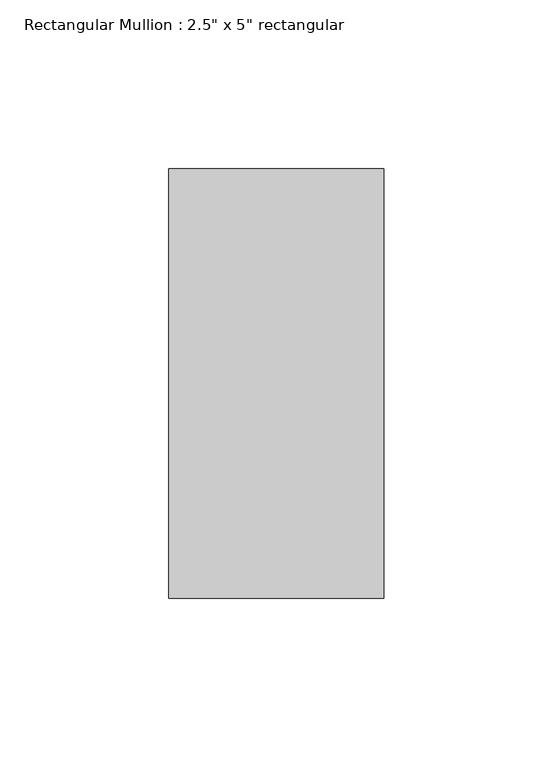
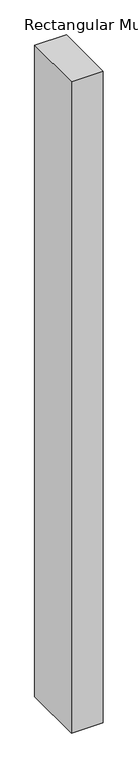
"""IFC4 building model written with IfcOpenShell, lengths in millimetres: member geometry."""

from ifc_helpers import new_model, si_unit, frame, origin, place, context, project, spatial, polyline, outline, extrude, source, transform, mapped, element, save


def member_f68f0f88(model_context):
    return source(origin(), model_context, "Body", "SweptSolid", [
        extrude(outline(polyline([(31.75, 63.5), (31.75, -63.5), (-31.75, -63.5), (-31.75, 63.5), (31.75, 63.5)])), frame((0.0, 0.0, -1376.6336497), z_axis=(0.0, 0.0, 1.0), x_axis=(1.0, 0.0, 0.0)), (0.0, 0.0, 1.0), 1376.6336497),
    ])


if __name__ == "__main__":
    model = new_model("IFC4")
    model_context = context("Model", 3, world=origin())
    ifc_project = project(units=[si_unit("LENGTHUNIT", "METRE", prefix="MILLI")], contexts=[model_context])
    site = spatial("IfcSite", under=ifc_project)
    building = spatial("IfcBuilding", under=site)
    placement = place(None, origin())
    member_shape = member_f68f0f88(model_context)
    element("IfcMember", 1, ObjectType="Rectangular Mullion : 2.5\" x 5\" rectangular", at=placement, inside=building, context=model_context, shape_type="MappedRepresentation", body=[
        mapped(member_shape, transform((0.0, 0.0, 0.0), x_axis=(1.0, 0.0, 0.0), y_axis=(0.0, 1.0, 0.0), z_axis=(0.0, 0.0, 1.0))),
    ])
    save(model, "model.ifc")

# Revit data of these elements
# Type "Rectangular Mullion : 2.5\" x 5\" rectangular"
#   built-in parameter 1007304 = 0.416667 (stored number, unit not read)
#   built-in parameter 1007301 = 0.104167 (stored number, unit not read)
#   built-in parameter 1007300 = 0.104167 (stored number, unit not read)
# Element 1 (IfcMember, "Rectangular Mullion : 2.5\" x 5\" rectangular")
#   Materials on its faces: "Aluminum"
# Materials
#   "Aluminum": class "Metal", colour RGB 247 247 247, transparency 0, Description = "Aluminum 6061", Cost = 0
